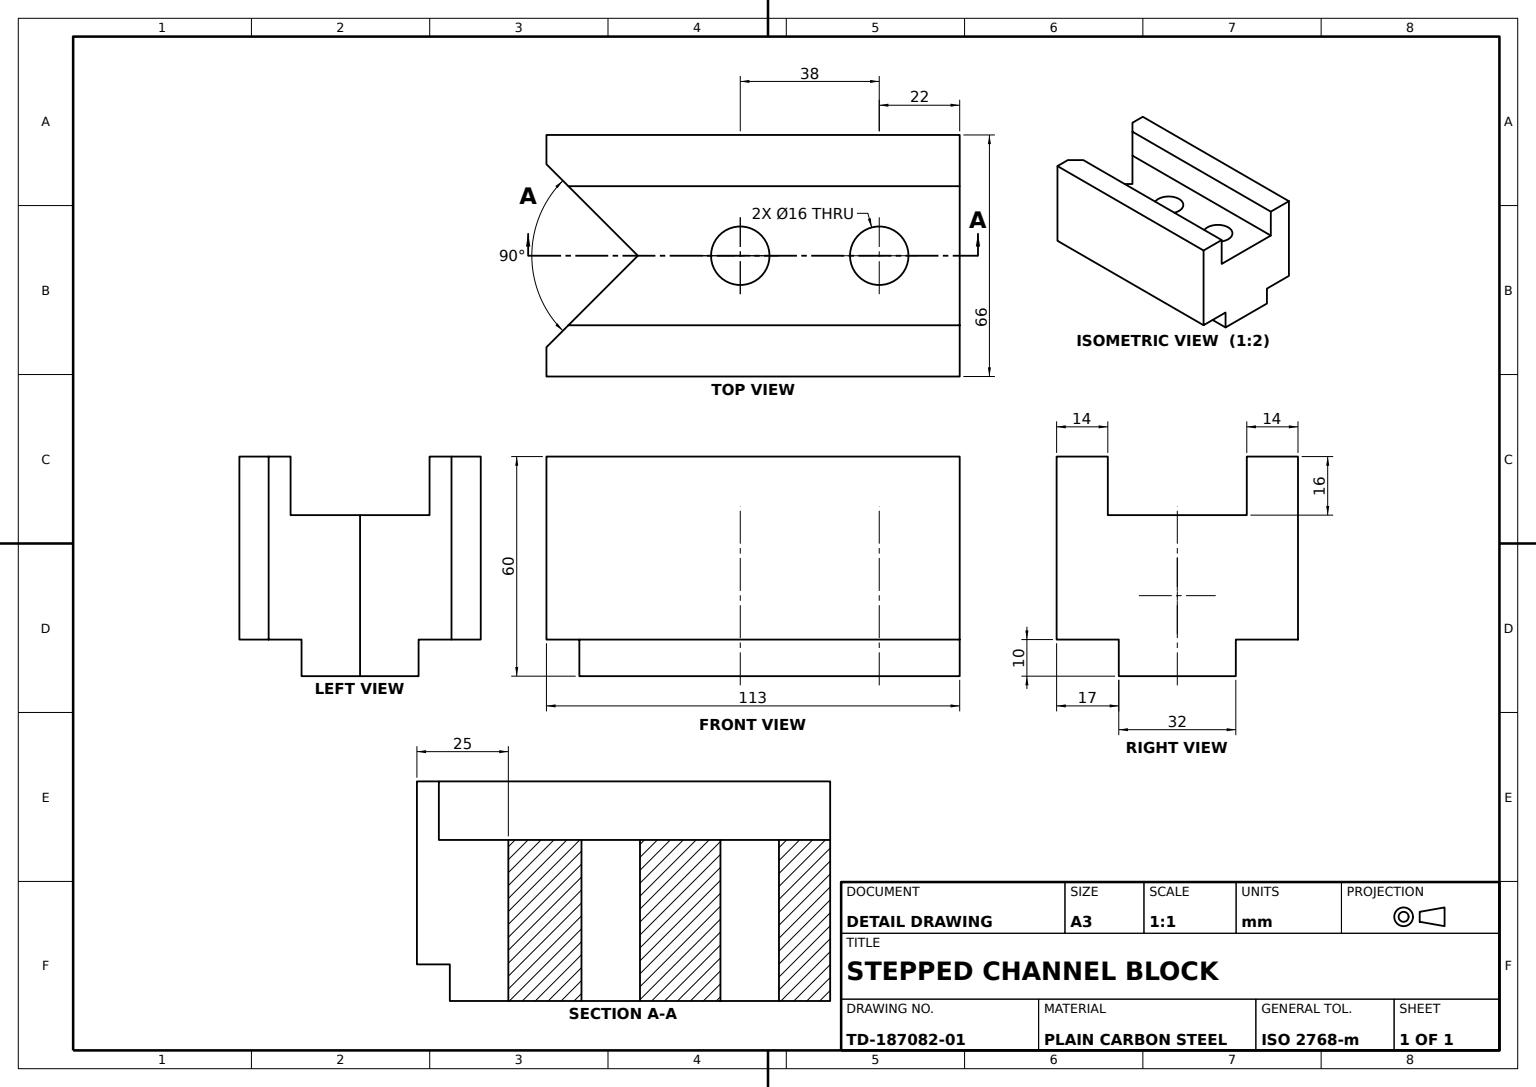
SolidWorks part; units mm, degrees
material "Plain Carbon Steel"
ref_plane "Front Plane" through (0, 0, 0) normal (0, 0, 1) x (1, 0, 0)
ref_plane "Top Plane" through (0, 0, 0) normal (0, 1, 0) x (1, 0, 0)
ref_plane "Right Plane" through (0, 0, 0) normal (1, 0, 0) x (0, 0, -1)
sketch "Channel Profile Sketch" plane through (0, 0, 0) normal (0, 0, 1) x (1, 0, 0)
  line L0 (0, 0) -> (0, 50)
  line L1 (0, 50) -> (14, 50)
  line L2 (14, 50) -> (14, 34)
  line L3 (14, 34) -> (52, 34)
  line L4 (52, 34) -> (52, 50)
  line L5 (52, 50) -> (66, 50)
  line L6 (66, 50) -> (66, 0)
  line L7 (66, 0) -> (49, 0)
  line L8 (49, 0) -> (49, -10)
  line L9 (49, -10) -> (17, -10)
  line L10 (17, -10) -> (17, 0)
  line L11 (17, 0) -> (0, 0)
  dimension "D1" = 66
  dimension "D2" = 50
  dimension "D3" = 14
  dimension "D4" = 16
  dimension "D5" = 10
  dimension "D6" = 32
extrude "Channel Block" add sketch "Channel Profile Sketch" along normal mid plane 113
sketch "Through Holes Sketch" plane through (0, 34, 0) normal (0, 1, 0) x (1, 0, 0)
  line L0 (52, 56.5) -> (14, 56.5) construction
  circle A0 centre (33, 34.5) radius 8
  circle A1 centre (33, -3.5) radius 8
  point P6 (33, 56.5)
  dimension "D1" = 16
  dimension "D2" = 22
  dimension "D3" = 38
extrude "Through Holes 2xØ16" cut sketch "Through Holes Sketch" against normal through all
sketch "Side Cut Sketch" plane through (0, 0, 0) normal (0, 1, 0) x (1, 0, 0)
  line L0 (8, -56.5) -> (33, -31.5)
  line L2 (33, -31.5) -> (58, -56.5)
  line L4 (52, -56.5) -> (14, -56.5) construction
  line L5 (66, -56.5) -> (52, -56.5) construction
  line L6 (14, -56.5) -> (0, -56.5) construction
  point P9 (33, -56.5)
  dimension "D1" = 90
  dimension "D2" = 25
extrude "Side Cut" cut sketch "Side Cut Sketch" against normal through all both and the other way through all flip side to cut
